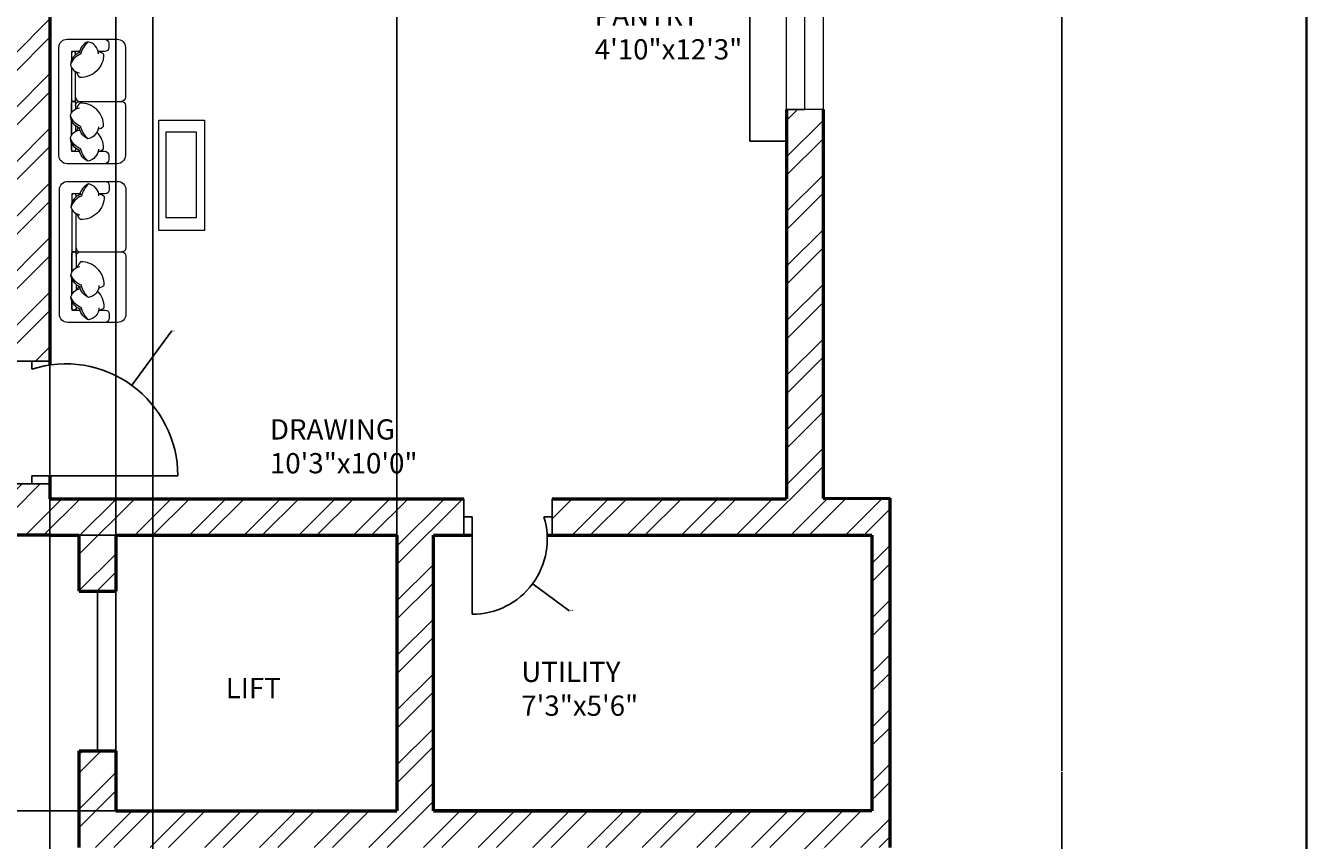
# Model space of a CAD drawing. Units: inches. Extents: x 1896 to 2572, y 1528 to 2474.
# Tile 9 of 10: x 2256 to 2572, y 2033 to 2234. Entities that reach past the tile are written whole.
import ezdxf

# ---------------------------------------------------------------- set-up
doc = ezdxf.new("R2010")
doc.units = ezdxf.units.IN
for name, color, linetype, lineweight in [('A-ANNO-DIMS', 2, 'Continuous', 18), ('A-ANNO-TTLB', 7, 'Continuous', 35), ('A-AREA-IDEN', 7, 'Continuous', 18), ('A-DOOR', 11, 'Continuous', 25), ('A-FLOR-CASE', 7, 'Continuous', 25), ('A-FURN', 8, 'Continuous', 18), ('A-GLAZ', 131, 'Continuous', 20), ('A-WALL', 7, 'Continuous', 50)]:
    doc.layers.add(name, color=color, linetype=linetype, lineweight=lineweight)
doc.layers.add('A-WALL-PATT', color=215, linetype='Continuous', lineweight=13, true_color=0xa953a0)
doc.styles.get("Standard").update_dxf_attribs({"font": 'arial.ttf'})
doc.dimstyles.get("Standard").update_dxf_attribs({"dimtxt": 0.18, "dimasz": 0.18, "dimexe": 0.18, "dimexo": 0.0625, "dimgap": 0.09, "dimtad": 0, "dimtih": 1, "dimtoh": 1, "dimdec": 4, "dimzin": 0, "dimdsep": 46, "dimtxsty": 'Standard', "dimcen": 0.09, "dimadec": 0, "dimazin": 0, "dimtfac": 1, "dimtdec": 4, "dimtofl": 0, "dimtmove": 0, "dimatfit": 3, "dimfxl": 1, "dimtolj": 1, "dimtzin": 0, "dimarcsym": 0})

# ---------------------------------------------------------------- blocks, each defined once
blk = doc.blocks.new('TABLE-COFFEE')
for points in [[(11.21, 0), (0, 0), (0, 27.27), (11.21, 27.27)], [(9.42, 2.87), (2.04, 2.87), (2.04, 24.13), (9.42, 24.13)]]:
    blk.add_lwpolyline(points, close=True)
blk = doc.blocks.new('WIN-36IN')
for p, q in [((0, 36), (9, 36)), ((0, 0), (0, 36)), ((9, 36), (4.5, 36)), ((4.5, 36), (4.5, 0)), ((9, 36), (9, 0)), ((4.5, 0), (0, 0)), ((0, 0), (9, 0))]:
    blk.add_line(p, q)
blk = doc.blocks.new('*D20')
at = {"layer": 'A-ANNO-DIMS', "color": 0, "lineweight": -2, "transparency": 16777216}
for p, q in [((2180.68, 2431.4), (2511.65, 2431.4)), ((2511.47, 2431.22), (2511.47, 2049.83)), ((2511.47, 1668.08), (2511.47, 2049.47)), ((2452.68, 1667.9), (2511.65, 1667.9))]:
    blk.add_line(p, q, dxfattribs=at)
at = {"layer": 'A-ANNO-DIMS', "color": 0, "transparency": 16777216}
for points in [[(2511.44, 2431.22), (2511.5, 2431.22), (2511.47, 2431.4)], [(2511.44, 1668.08), (2511.5, 1668.08), (2511.47, 1667.9)]]:
    blk.add_solid(points, dxfattribs=at)
at = {"layer": 'Defpoints', "color": 0, "transparency": 16777216}
for p in [(2180.62, 2431.4), (2511.47, 2431.4), (2452.62, 1667.9)]:
    blk.add_point(p, dxfattribs=at)
at = {"layer": 'A-ANNO-DIMS', "color": 0, "transparency": 16777216, "insert": (2511.47, 2049.65), "char_height": 0.18, "attachment_point": 5}
blk.add_mtext('\\A1;763.5', dxfattribs=at)
blk = doc.blocks.new('*D29')
at = {"layer": 'A-ANNO-DIMS', "color": 0, "lineweight": -2, "transparency": 16777216}
for p, q in [((2278.35, 2039.96), (2278.35, 2473.93)), ((2278.53, 2473.75), (2312.59, 2473.75)), ((2347.44, 2473.75), (2313.38, 2473.75)), ((2347.62, 2039.96), (2347.62, 2473.93))]:
    blk.add_line(p, q, dxfattribs=at)
at = {"layer": 'A-ANNO-DIMS', "color": 0, "transparency": 16777216}
for points in [[(2278.53, 2473.78), (2278.53, 2473.72), (2278.35, 2473.75)], [(2347.44, 2473.78), (2347.44, 2473.72), (2347.62, 2473.75)]]:
    blk.add_solid(points, dxfattribs=at)
at = {"layer": 'Defpoints', "color": 0, "transparency": 16777216}
for p in [(2347.62, 2473.75), (2278.35, 2039.9), (2347.62, 2039.9)]:
    blk.add_point(p, dxfattribs=at)
at = {"layer": 'A-ANNO-DIMS', "color": 0, "transparency": 16777216, "insert": (2312.99, 2473.75), "char_height": 0.18, "attachment_point": 5}
blk.add_mtext('\\A1;69.27', dxfattribs=at)
blk = doc.blocks.new('*D30')
at = {"layer": 'A-ANNO-DIMS', "color": 0, "lineweight": -2, "transparency": 16777216}
for p, q in [((2347.56, 2107.9), (1919.59, 2107.9)), ((1919.77, 2107.72), (1919.77, 2074.08)), ((1919.77, 2040.08), (1919.77, 2073.72)), ((2347.56, 2039.9), (1919.59, 2039.9))]:
    blk.add_line(p, q, dxfattribs=at)
at = {"layer": 'A-ANNO-DIMS', "color": 0, "transparency": 16777216}
for points in [[(1919.74, 2107.72), (1919.8, 2107.72), (1919.77, 2107.9)], [(1919.74, 2040.08), (1919.8, 2040.08), (1919.77, 2039.9)]]:
    blk.add_solid(points, dxfattribs=at)
at = {"layer": 'Defpoints', "color": 0, "transparency": 16777216}
for p in [(1919.77, 2107.9), (2347.62, 2107.9), (2347.62, 2039.9)]:
    blk.add_point(p, dxfattribs=at)
at = {"layer": 'A-ANNO-DIMS', "color": 0, "transparency": 16777216, "insert": (1919.77, 2073.9), "char_height": 0.18, "attachment_point": 5}
blk.add_mtext('\\A1;68', dxfattribs=at)
blk = doc.blocks.new('*D35')
at = {"layer": 'A-ANNO-DIMS', "color": 0, "lineweight": -2, "transparency": 16777216}
for p, q in [((2262.12, 2373.34), (2262.12, 1549.1)), ((2287.46, 2373.34), (2287.46, 1549.1)), ((2262.3, 1549.28), (2274.4, 1549.28)), ((2287.28, 1549.28), (2275.19, 1549.28))]:
    blk.add_line(p, q, dxfattribs=at)
at = {"layer": 'A-ANNO-DIMS', "color": 0, "transparency": 16777216}
for points in [[(2262.3, 1549.31), (2262.3, 1549.25), (2262.12, 1549.28)], [(2287.28, 1549.31), (2287.28, 1549.25), (2287.46, 1549.28)]]:
    blk.add_solid(points, dxfattribs=at)
at = {"layer": 'Defpoints', "color": 0, "transparency": 16777216}
for p in [(2262.12, 2373.4), (2287.46, 2373.4), (2287.46, 1549.28)]:
    blk.add_point(p, dxfattribs=at)
at = {"layer": 'A-ANNO-DIMS', "color": 0, "transparency": 16777216, "insert": (2274.79, 1549.28), "char_height": 0.18, "attachment_point": 5}
blk.add_mtext('\\A1;25.34', dxfattribs=at)
blk = doc.blocks.new('*D41')
at = {"layer": 'A-ANNO-DIMS', "color": 0, "lineweight": -2, "transparency": 16777216}
for p, q in [((2292.07, 2158.2), (2282.41, 2144.97)), ((2292.25, 2158.2), (2292.07, 2158.2)), ((2265.93, 2122.54), (2266.11, 2122.54)), ((2266.02, 2122.45), (2266.02, 2122.63))]:
    blk.add_line(p, q, dxfattribs=at)
at = {"layer": 'A-ANNO-DIMS', "color": 0, "transparency": 16777216}
blk.add_solid([(2282.38, 2144.99), (2282.43, 2144.96), (2282.3, 2144.83)], dxfattribs=at)
at = {"layer": 'Defpoints', "color": 0, "transparency": 16777216}
for p in [(2282.3, 2144.83), (2266.02, 2122.54)]:
    blk.add_point(p, dxfattribs=at)
at = {"layer": 'A-ANNO-DIMS', "color": 0, "transparency": 16777216, "insert": (2292.66, 2158.2), "char_height": 0.18, "attachment_point": 5}
blk.add_mtext('\\A1;R27.6', dxfattribs=at)
blk = doc.blocks.new('*D49')
at = {"layer": 'A-ANNO-DIMS', "color": 0, "lineweight": -2, "transparency": 16777216}
for p, q in [((2366.04, 2106.93), (2366.22, 2106.93)), ((2366.13, 2106.84), (2366.13, 2107.02)), ((2389.99, 2089.33), (2381.18, 2095.82)), ((2390.17, 2089.33), (2389.99, 2089.33))]:
    blk.add_line(p, q, dxfattribs=at)
at = {"layer": 'A-ANNO-DIMS', "color": 0, "transparency": 16777216}
blk.add_solid([(2381.2, 2095.85), (2381.17, 2095.8), (2381.04, 2095.93)], dxfattribs=at)
at = {"layer": 'Defpoints', "color": 0, "transparency": 16777216}
for p in [(2366.13, 2106.93), (2381.04, 2095.93)]:
    blk.add_point(p, dxfattribs=at)
at = {"layer": 'A-ANNO-DIMS', "color": 0, "transparency": 16777216, "insert": (2390.65, 2089.33), "char_height": 0.18, "attachment_point": 5}
blk.add_mtext('\\A1;R18.53', dxfattribs=at)

msp = doc.modelspace()

# ---------------------------------------------------------------- hatches: boundary and pattern name
at = {"layer": 'A-WALL-PATT'}
h = msp.add_hatch(dxfattribs=at)
h.set_pattern_fill('ANSI32', color=256)
h.paths.add_polyline_path([(2071.6224, 2382.3979), (2071.6224, 2422.3979), (2110.6224, 2422.3979), (2110.6224, 2382.3979), (2110.6224, 2357.5961), (2119.6224, 2357.5961), (2119.6224, 2422.3979), (2171.6224, 2422.3979), (2171.6224, 2373.3979), (2193.5093, 2373.3979), (2193.5093, 2377.8979), (2193.5093, 2382.3979), (2180.6224, 2382.3979), (2180.6224, 2431.3979), (2171.6224, 2431.3979), (2119.6224, 2431.3979), (2110.6224, 2431.3979), (2062.6224, 2431.3979), (2062.6224, 2422.3979), (2062.6224, 2382.3979), (1978.6224, 2382.3979), (1978.6224, 2313.0337), (1987.6224, 2313.0337), (1987.6224, 2373.3979), (2062.6224, 2373.3979), (2067.1224, 2373.3979), (2067.1224, 2353.7982), (2071.6224, 2353.8883)])
h.paths.add_polyline_path([(2287.4624, 2382.3979), (2229.5093, 2382.3979), (2229.5093, 2373.3979), (2253.1224, 2373.3979), (2253.1224, 2175.8979), (2247.1039, 2175.8979), (2247.1039, 2166.8979), (2253.1224, 2166.8979), (2253.1224, 2150.8283), (2262.1224, 2150.8283), (2262.1224, 2166.8979), (2262.1224, 2236.8979), (2349.0731, 2236.8979), (2349.0731, 2239.1479), (2349.0731, 2241.3979), (2262.1224, 2241.3979), (2262.1224, 2373.3979), (2287.4624, 2373.3979)])
h.paths.add_polyline_path([(2452.6224, 2382.3979), (2347.4624, 2382.3979), (2347.4624, 2373.3979), (2382.1224, 2373.3979), (2382.1224, 2334.0335), (2386.6224, 2334.0335), (2386.6224, 2373.3979), (2443.6224, 2373.3979), (2443.6224, 2316.2056), (2452.6224, 2316.2056)])
h.paths.add_polyline_path([(2452.6224, 2292.2056), (2448.1224, 2292.2056), (2443.6224, 2292.2056), (2443.6224, 2292.0047), (2443.6224, 2280.9372), (2443.6224, 2268.3979), (2386.6224, 2268.3979), (2386.6224, 2312.4044), (2384.3724, 2312.4044), (2382.1224, 2312.4044), (2382.1224, 2241.3979), (2379.1336, 2241.3979), (2379.1336, 2236.8979), (2386.6224, 2236.8979), (2386.6224, 2263.8979), (2443.6224, 2263.8979), (2443.6224, 2248.8449), (2452.6224, 2248.8449)])
h.paths.add_polyline_path([(2364.1285, 2116.8979), (2262.1224, 2116.8979), (2262.1224, 2120.5401), (2257.6224, 2120.5401), (2253.1224, 2120.5401), (2253.1224, 2107.8979), (2262.1224, 2107.8979), (2269.354, 2107.8979), (2269.354, 2094.0702), (2278.354, 2094.0702), (2278.354, 2107.8979), (2347.6224, 2107.8979), (2347.6224, 2039.8979), (2278.354, 2039.8979), (2278.354, 2054.7605), (2269.354, 2054.7605), (2269.354, 2030.8979), (2278.354, 2030.8979), (2443.6224, 2030.8979), (2443.6224, 2015.198), (2452.6224, 2015.198), (2452.6224, 2030.8979), (2464.6224, 2030.8979), (2469.1224, 2030.8979), (2469.1224, 2117.0352), (2452.6767, 2116.9466), (2452.6285, 2125.8979), (2452.6224, 2125.8979), (2452.6224, 2212.8449), (2443.6224, 2212.8449), (2443.6224, 2116.8979), (2385.832, 2116.8979), (2385.832, 2112.3979), (2385.832, 2107.8979), (2464.6224, 2107.8979), (2464.6224, 2039.8979), (2443.6224, 2039.8979), (2356.6224, 2039.8979), (2356.6224, 2107.8979), (2364.1285, 2107.8979)])
h.paths.add_polyline_path([(2452.6224, 1967.198), (2443.6224, 1967.198), (2443.6224, 1955.8979), (2259.1224, 1955.8979), (2254.6224, 1955.8979), (2254.6224, 1941.6358), (2263.6224, 1941.6358), (2263.6224, 1946.8979), (2379.1224, 1946.8979), (2379.1224, 1913.0204), (2383.6224, 1913.0204), (2383.6224, 1946.8979), (2443.6224, 1946.8979), (2443.6224, 1930.729), (2452.6224, 1930.729)])
h.paths.add_polyline_path([(2469.1224, 1871.8979), (2464.6224, 1871.8979), (2452.6224, 1871.8979), (2452.6224, 1894.729), (2443.6224, 1894.729), (2443.6224, 1871.8979), (2388.1304, 1871.8979), (2388.1304, 1867.3979), (2443.6224, 1867.3979), (2464.6224, 1867.3979), (2464.6224, 1817.8979), (2443.6224, 1817.8979), (2388.1304, 1817.8979), (2388.1304, 1815.6479), (2388.1304, 1813.3979), (2391.1224, 1813.3979), (2391.1224, 1747.8899), (2395.6224, 1747.8899), (2395.6224, 1813.3979), (2443.6224, 1813.3979), (2443.6224, 1781.4434), (2452.6224, 1781.4434), (2452.6224, 1813.3979), (2464.6224, 1813.3979), (2469.1224, 1813.3979)])
h.paths.add_polyline_path([(2263.6224, 1910.9737), (2259.1224, 1910.9737), (2254.6224, 1910.9737), (2254.6224, 1889.8979), (2251.2778, 1889.8979), (2251.2778, 1880.8979), (2254.6224, 1880.8979), (2254.6224, 1817.8979), (2254.6224, 1754.8979), (2254.6224, 1693.3979), (2254.6224, 1684.3979), (2254.6224, 1672.3979), (2200.6224, 1672.3979), (2200.6224, 1684.3979), (2200.6224, 1693.3979), (2200.6224, 1754.8979), (2196.1224, 1754.8979), (2196.1224, 1693.3979), (2150.0488, 1693.3979), (2150.0488, 1684.3979), (2196.1224, 1684.3979), (2196.1224, 1672.3979), (2196.1224, 1667.8979), (2254.6224, 1667.8979), (2259.1224, 1667.8979), (2259.1224, 1693.3979), (2259.1224, 1813.3979), (2353.6224, 1813.3979), (2353.6224, 1815.6479), (2353.6224, 1817.8979), (2263.6224, 1817.8979)])
h.paths.add_polyline_path([(2391.1224, 1693.3979), (2345.6981, 1693.3979), (2345.6981, 1684.3979), (2391.1224, 1684.3979)])
h.paths.add_polyline_path([(2285.6981, 1693.3979), (2259.1224, 1693.3979), (2259.1224, 1684.3979), (2285.6981, 1684.3979), (2285.6981, 1688.8979)], flags=17)
h.paths.add_polyline_path([(2452.6224, 1757.4434), (2448.1224, 1757.4434), (2443.6224, 1757.4434), (2443.6224, 1726.3979), (2395.6224, 1726.3979), (2395.6224, 1728.6572), (2393.3724, 1728.6572), (2391.1224, 1728.6572), (2391.1224, 1717.6723), (2395.6224, 1717.6723), (2395.6224, 1721.8979), (2443.6224, 1721.8979), (2443.6224, 1714.8), (2452.6224, 1714.8)])
h.paths.add_polyline_path([(2452.6224, 1684.3979), (2452.6224, 1690.8), (2443.6224, 1690.8), (2443.6224, 1679.8979), (2443.6224, 1672.3979), (2395.6224, 1672.3979), (2395.6224, 1695.6708), (2391.1224, 1695.5986), (2391.1224, 1672.3979), (2391.1224, 1667.8979), (2452.6224, 1667.8979)])
h.paths.add_polyline_path([(1987.6224, 1880.8979), (2068.6224, 1880.8979), (2125.6224, 1880.8979), (2125.6224, 1788.8466), (2130.1224, 1788.8466), (2130.1224, 1880.8979), (2216.1958, 1880.8979), (2216.1958, 1885.3979), (2216.1958, 1889.8979), (2208.1224, 1889.8979), (2208.1224, 1996.3717), (2203.6224, 1996.3717), (2199.1224, 1996.3717), (2199.1224, 1889.8979), (2073.1224, 1889.8979), (2073.1224, 1917.1874), (2068.6224, 1917.1874), (2068.6224, 1889.8979), (1987.6224, 1889.8979), (1987.6224, 1912.4976), (1978.6224, 1912.4976), (1978.6224, 1805.5193), (1987.6224, 1805.5193)])
h.paths.add_polyline_path([(2019.9303, 1754.8979), (1987.6224, 1754.8979), (1966.6224, 1754.8979), (1966.6224, 1801.0193), (1987.6224, 1801.0193), (1987.6224, 1805.5193), (1962.1224, 1805.5193), (1962.1224, 1750.3979), (1966.6224, 1750.3979), (1978.6224, 1750.3979), (1987.6224, 1750.3979), (2019.9303, 1750.3979)])
h.paths.add_polyline_path([(2135.5566, 1754.8979), (2130.1224, 1754.8979), (2130.1224, 1758.052), (2127.8724, 1758.052), (2125.6224, 1758.052), (2125.6224, 1754.8979), (2068.6224, 1754.8979), (2043.2292, 1754.8979), (2043.2292, 1750.3979), (2068.6224, 1750.3979), (2098.6224, 1750.3979), (2098.6224, 1693.3979), (2068.6224, 1693.3979), (1987.6224, 1693.3979), (1987.6224, 1707.3003), (1983.1224, 1707.3003), (1978.6224, 1707.3003), (1978.6224, 1684.3979), (2068.6224, 1684.3979), (2126.0488, 1684.3979), (2126.0488, 1688.8979), (2126.0488, 1693.3979), (2103.1224, 1693.3979), (2103.1224, 1750.3979), (2130.1224, 1750.3979), (2135.5566, 1750.3979)])
h.paths.add_polyline_path([(1987.6224, 1750.3979), (1978.6224, 1750.3979), (1978.6224, 1731.3003), (1987.6224, 1731.3003)], flags=0)
h.paths.add_polyline_path([(1987.6224, 1973.8979), (2068.6224, 1973.8979), (2073.1224, 1973.8979), (2073.1224, 1978.3979), (1971.1224, 1978.3979), (1971.1224, 2030.3979), (1978.6224, 2030.3979), (1987.6224, 2030.3979), (2104.9199, 2030.3979), (2104.9199, 2032.6479), (2104.9199, 2034.8979), (1987.6224, 2034.8979), (1971.1224, 2034.8979), (1971.1224, 2085.8979), (2003.6464, 2085.8979), (2003.6464, 2090.3979), (1987.6224, 2090.3979), (1987.6224, 2166.8979), (2115.1224, 2166.8979), (2137.6224, 2166.8979), (2137.6224, 2114.4229), (2142.1224, 2114.4229), (2142.1224, 2124.8979), (2153.5306, 2124.8979), (2153.5306, 2127.1479), (2153.5306, 2129.3979), (2142.1224, 2129.3979), (2142.1224, 2166.8979), (2199.1224, 2166.8979), (2199.1224, 2129.3979), (2177.5306, 2129.3979), (2177.5306, 2124.8979), (2199.1224, 2124.8979), (2199.1224, 2034.8979), (2142.1224, 2034.8979), (2142.1224, 2091.6671), (2139.8724, 2091.6671), (2137.6224, 2091.6671), (2137.6224, 2034.8979), (2133.8326, 2034.8979), (2133.8326, 2030.3979), (2137.6224, 2030.3979), (2142.1224, 2030.3979), (2199.1224, 2030.3979), (2199.1224, 2024.2654), (2208.1224, 2024.2654), (2208.1224, 2030.3979), (2208.1224, 2166.8979), (2214.5775, 2166.8979), (2214.5775, 2171.3979), (2214.5775, 2175.8979), (2115.1224, 2175.8979), (2115.1224, 2329.9154), (2112.4137, 2329.9154), (2110.6224, 2329.9154), (2110.6224, 2175.8979), (2082.1224, 2175.8979), (2082.1224, 2202.6443), (2079.8724, 2202.6443), (2077.6224, 2202.6443), (2077.6224, 2175.8979), (1987.6224, 2175.8979), (1987.6224, 2191.3531), (1983.1224, 2191.3531), (1978.6224, 2191.3531), (1978.6224, 2090.3979), (1966.6224, 2090.3979), (1966.6224, 2085.8979), (1966.6224, 2030.3979), (1966.6224, 1973.8979), (1978.6224, 1973.8979), (1978.6224, 1948.4976), (1983.1224, 1948.4976), (1987.6224, 1948.4976)])
h.paths.add_polyline_path([(1987.6224, 2253.0337), (1983.1224, 2253.0337), (1978.6224, 2253.0337), (1978.6224, 2215.3531), (1987.6224, 2215.3531), (1987.6224, 2224.8979), (2077.6224, 2224.8979), (2077.6224, 2221.9854), (2082.1224, 2221.9854), (2082.1224, 2229.3979), (1987.6224, 2229.3979)], flags=17)
h.paths.add_polyline_path([(2220.5047, 1978.7278), (2253.7278, 1978.7278), (2253.7278, 1997.3851), (2220.5047, 1997.3851)], flags=9)
h.paths.add_polyline_path([(2303.6746, 2064.9806), (2320.5334, 2064.9806), (2320.5334, 2075.2842), (2303.6746, 2075.2842)], flags=25)

# ---------------------------------------------------------------- linework, layer by layer
at = {"layer": 'A-ANNO-TTLB'}
msp.add_lwpolyline([(1895.84, 2455.9668), (2571.702, 2455.9668), (2571.702, 1527.8833), (1895.84, 1527.8833)], close=True, dxfattribs=at)
at = {"layer": 'A-DOOR'}
for p, q in [((2253.1224, 2150.8283), (2262.1224, 2150.8283)), ((2262.1224, 2150.8283), (2257.6224, 2150.8283)), ((2257.6224, 2150.8283), (2257.6224, 2148.8283)), ((2257.6224, 2120.5401), (2257.6224, 2122.5401)), ((2257.6224, 2122.5401), (2293.6224, 2122.5401)), ((2253.1224, 2120.5401), (2262.1224, 2120.5401)), ((2262.1224, 2120.5401), (2257.6224, 2120.5401)), ((2364.1285, 2107.8979), (2364.1285, 2116.8979)), ((2364.1285, 2116.8979), (2364.1285, 2112.3979)), ((2385.832, 2107.8979), (2385.832, 2116.8979)), ((2385.832, 2116.8979), (2385.832, 2116.8979)), ((2385.832, 2116.8979), (2385.832, 2112.3979)), ((2364.1285, 2112.3979), (2366.1285, 2112.3979)), ((2366.1285, 2112.3979), (2366.1285, 2088.3979)), ((2385.832, 2112.3979), (2383.832, 2112.3979)), ((2273.854, 2094.0702), (2273.854, 2054.7605))]:
    msp.add_line(p, q, dxfattribs=at)
for centre, radius, start, end in [((2266.0243, 2122.5401), 27.5982, 0, 107.724107), ((2366.1285, 2106.9274), 18.5295, 270, 17.171415)]:
    msp.add_arc(centre, radius, start, end, dxfattribs=at)
at = {"layer": 'A-FLOR-CASE'}
for p, q in [((2434.5516, 2255.5451), (2434.5516, 2205.0449)), ((2434.5516, 2205.0449), (2443.6224, 2205.0449))]:
    msp.add_line(p, q, dxfattribs=at)
at = {"layer": 'A-FURN', "ltscale": 0.03}
for points in [[(2280.7017, 2215.8729, -0.41421356), (2279.6783, 2214.8495, -0.41421356), (2280.7017, 2213.8261), (2280.7017, 2201.5452, -0.41421356), (2278.6549, 2199.4984), (2266.374, 2199.4984, -0.41421356), (2264.3272, 2201.5452), (2264.3272, 2228.1538, -0.41421356), (2266.374, 2230.2006), (2278.6549, 2230.2006, -0.41421356), (2280.7017, 2228.1538), (2280.7017, 2215.8729, -0.41421356), (2279.6783, 2214.8495, -0.41421356), (2280.7017, 2213.8261)], [(2280.8392, 2178.7738, -0.41421356), (2279.8158, 2177.7504, -0.41421356), (2280.8392, 2176.727), (2280.8392, 2162.3993, -0.41421356), (2278.7924, 2160.3525), (2266.5115, 2160.3525, -0.41421356), (2264.4647, 2162.3993), (2264.4647, 2193.1016, -0.41421356), (2266.5115, 2195.1484), (2278.7924, 2195.1484, -0.41421356), (2280.8392, 2193.1016), (2280.8392, 2178.7738, -0.41421356), (2279.8158, 2177.7504, -0.41421356), (2280.8392, 2176.727)]]:
    msp.add_lwpolyline(points, format="xyb", dxfattribs=at)
at = {"layer": 'A-FURN'}
for points in [[(2271.4814, 2229.5493, 0.14772988), (2269.7225, 2226.5581, 0.21334276), (2267.1429, 2223.9189, 0.17866181)], [(2274.061, 2226.6168, 0.35677236), (2271.4814, 2229.5493, 0.24954205), (2269.3555, 2226.8922, -9.61688035)], [(2275.5847, 2230.2006, -0.41421356), (2276.6081, 2229.1772), (2276.6081, 2228.1538, -0.41421356), (2275.5847, 2227.1304), (2273.9991, 2227.1304)], [(2269.5824, 2226.9714, 0.30666349), (2267.1429, 2223.9189, 0.30632997), (2269.3708, 2221.9248, -0.87284716)], [(2268.4208, 2226.3494), (2268.4208, 2226.721, 0.41421356), (2268.0115, 2227.1304), (2267.8068, 2227.1304, 0.41421356), (2267.3974, 2226.721)], [(2267.3974, 2226.721), (2267.3974, 2224.9774, 0.41421356)], [(2273.9986, 2227.1326, -0.16554063), (2275.3508, 2226.4995, -0.42598917), (2269.488, 2220.7518, -0.12152332), (2268.68, 2222.1162, 7.11546429)], [(2267.3974, 2223.2748), (2267.3974, 2215.2589, 0.41421356), (2267.8068, 2214.8495), (2268.0115, 2214.8495, 0.41421356), (2268.4208, 2215.2589), (2268.4208, 2222.2443, 0.41421356)], [(2268.4208, 2215.8729, 0.41421356), (2269.4442, 2214.8495)], [(2268.4208, 2215.8729, 0.41421356), (2269.4442, 2214.8495), (2279.6783, 2214.8495, 0.41421356)], [(2269.5824, 2208.2407, -0.30666349), (2267.1429, 2211.2931, -0.30632997), (2269.3708, 2213.2872, 0.87284716)], [(2267.3974, 2211.9372), (2267.3974, 2214.4401, -0.41421356), (2267.8068, 2214.8495), (2268.0115, 2214.8495, -0.41421356), (2268.4208, 2214.4401), (2268.4208, 2212.9677, -0.41421356)], [(2268.4208, 2213.8261, -0.41421356), (2269.4442, 2214.8495)], [(2268.4208, 2213.8261, -0.41421356), (2269.4442, 2214.8495), (2279.6783, 2214.8495, -0.41421356)], [(2273.9986, 2208.0794, 0.16554063), (2275.3508, 2208.7125, 0.42598917), (2269.488, 2214.4602, 0.12152332), (2268.68, 2213.0958, -7.11546429)], [(2271.4814, 2205.6628, -0.14772988), (2269.7225, 2208.6539, -0.21334276), (2267.1429, 2211.2931, -0.17866181)], [(2267.3974, 2206.4241), (2267.3974, 2210.2346, -0.41421356)], [(2269.5824, 2202.7276, -0.30666349), (2267.1429, 2205.7801, -0.30632997), (2269.3708, 2207.7742, 0.87284716)], [(2268.4208, 2208.8626), (2268.4208, 2207.4547, -0.41421356)], [(2269.0801, 2208.4408, 0.07186538), (2268.68, 2207.5828, -7.11546429)], [(2274.061, 2208.5952, -0.35677236), (2271.4814, 2205.6628, -0.24954205), (2269.3555, 2208.3199, 9.61688035)], [(2273.9986, 2202.5664, 0.16554063), (2275.3508, 2203.1995, 0.20023115), (2273.7039, 2207.262, 0.12152332)], [(2271.4814, 2200.1497, -0.14772988), (2269.7225, 2203.1408, -0.21334276), (2267.1429, 2205.7801, -0.17866181)], [(2267.3974, 2202.978), (2267.3974, 2204.7216, -0.41421356)], [(2267.3974, 2204.7216), (2267.3974, 2202.5686), (2269.4087, 2202.5686, -0.41421356)], [(2268.4208, 2203.3496), (2268.4208, 2202.978, -0.41421356), (2268.0115, 2202.5686), (2267.8068, 2202.5686, -0.41421356), (2267.3974, 2202.978)], [(2274.061, 2203.0822, -0.35677236), (2271.4814, 2200.1497, -0.24954205), (2269.3555, 2202.8068, 9.61688035)], [(2273.9991, 2202.5686), (2275.5847, 2202.5686, -0.41421356), (2276.6081, 2201.5452), (2276.6081, 2200.5218, -0.41421356), (2275.5847, 2199.4984)], [(2271.6189, 2194.497, 0.14772988), (2269.86, 2191.5059, 0.21334276), (2267.2804, 2188.8667, 0.17866181)], [(2274.1985, 2191.5646, 0.35677236), (2271.6189, 2194.497, 0.24954205), (2269.493, 2191.8399, -9.61688035)], [(2275.7222, 2195.1484, -0.41421356), (2276.7456, 2194.125), (2276.7456, 2193.1016, -0.41421356), (2275.7222, 2192.0781), (2274.1365, 2192.0781)], [(2269.7199, 2191.9191, 0.30666349), (2267.2804, 2188.8667, 0.30632997), (2269.5083, 2186.8726, -0.87284716)], [(2268.5583, 2191.2972), (2268.5583, 2191.6688, 0.41421356), (2268.149, 2192.0781), (2267.9443, 2192.0781, 0.41421356), (2267.5349, 2191.6688)], [(2267.5349, 2191.6688), (2267.5349, 2189.9252, 0.41421356)], [(2274.1361, 2192.0804, -0.16554063), (2275.4883, 2191.4473, -0.42598917), (2269.6255, 2185.6996, -0.12152332), (2268.8174, 2187.064, 7.11546429)], [(2267.5349, 2188.2226), (2267.5349, 2178.1598, 0.41421356), (2267.9443, 2177.7504), (2268.149, 2177.7504, 0.41421356), (2268.5583, 2178.1598), (2268.5583, 2187.1921, 0.41421356)], [(2267.5349, 2172.7913), (2267.5349, 2177.3411, -0.41421356), (2267.9443, 2177.7504), (2268.149, 2177.7504, -0.41421356), (2268.5583, 2177.3411), (2268.5583, 2173.8218, -0.41421356)], [(2268.5583, 2178.7738, 0.41421356), (2269.5817, 2177.7504)], [(2268.5583, 2178.7738, 0.41421356), (2269.5817, 2177.7504), (2279.8158, 2177.7504, 0.41421356)], [(2268.5583, 2176.727, -0.41421356), (2269.5817, 2177.7504)], [(2268.5583, 2176.727, -0.41421356), (2269.5817, 2177.7504), (2279.8158, 2177.7504, -0.41421356)], [(2274.1361, 2168.9336, 0.16554063), (2275.4883, 2169.5667, 0.42598917), (2269.6255, 2175.3143, 0.12152332), (2268.8174, 2173.9499, -7.11546429)], [(2269.7199, 2169.0948, -0.30666349), (2267.2804, 2172.1473, -0.30632997), (2269.5083, 2174.1413, 0.87284716)], [(2271.6189, 2166.5169, -0.14772988), (2269.86, 2169.508, -0.21334276), (2267.2804, 2172.1473, -0.17866181)], [(2269.7199, 2163.5817, -0.30666349), (2267.2804, 2166.6342, -0.30632997), (2269.5083, 2168.6283, 0.87284716)], [(2267.5349, 2167.2783), (2267.5349, 2171.0888, -0.41421356)], [(2268.5583, 2169.7168), (2268.5583, 2168.3088, -0.41421356)], [(2269.2175, 2169.2949, 0.07186538), (2268.8174, 2168.4369, -7.11546429)], [(2274.1985, 2169.4494, -0.35677236), (2271.6189, 2166.5169, -0.24954205), (2269.493, 2169.174, 9.61688035)], [(2274.1361, 2163.4205, 0.16554063), (2275.4883, 2164.0536, 0.20023115), (2273.8414, 2168.1162, 0.12152332)], [(2271.6189, 2161.0038, -0.14772988), (2269.86, 2163.995, -0.21334276), (2267.2804, 2166.6342, -0.17866181)], [(2267.5349, 2165.5757), (2267.5349, 2163.4227), (2269.5462, 2163.4227, -0.41421356)], [(2267.5349, 2163.8321), (2267.5349, 2165.5757, -0.41421356)], [(2268.5583, 2164.2037), (2268.5583, 2163.8321, -0.41421356), (2268.149, 2163.4227), (2267.9443, 2163.4227, -0.41421356), (2267.5349, 2163.8321)], [(2274.1985, 2163.9363, -0.35677236), (2271.6189, 2161.0038, -0.24954205), (2269.493, 2163.6609, 9.61688035)], [(2274.1365, 2163.4227), (2275.7222, 2163.4227, -0.41421356), (2276.7456, 2162.3993), (2276.7456, 2161.3759, -0.41421356), (2275.7222, 2160.3525)]]:
    msp.add_lwpolyline(points, format="xyb", dxfattribs=at)
for points in [[(2269.4087, 2227.1304), (2267.3974, 2227.1304), (2267.3974, 2224.9774)], [(2267.3974, 2223.2748), (2267.3974, 2211.9372)], [(2267.3974, 2210.2346), (2267.3974, 2206.4241)], [(2269.5462, 2192.0781), (2267.5349, 2192.0781), (2267.5349, 2189.9252)], [(2267.5349, 2188.2226), (2267.5349, 2172.7913)], [(2267.5349, 2171.0888), (2267.5349, 2167.2783)]]:
    msp.add_lwpolyline(points, dxfattribs=at)
for points in [[(2267.3974, 2215.2589), (2267.3974, 2214.4401, -0.41421356), (2267.8068, 2214.8495), (2268.0115, 2214.8495, -0.41421356), (2268.4208, 2214.4401), (2268.4208, 2215.2589, -0.41421356), (2268.0115, 2214.8495), (2267.8068, 2214.8495, -0.41421356)], [(2267.5349, 2178.1598), (2267.5349, 2177.3411, -0.41421356), (2267.9443, 2177.7504), (2268.149, 2177.7504, -0.41421356), (2268.5583, 2177.3411), (2268.5583, 2178.1598, -0.41421356), (2268.149, 2177.7504), (2267.9443, 2177.7504, -0.41421356)]]:
    msp.add_lwpolyline(points, format="xyb", close=True, dxfattribs=at)
at = {"layer": 'A-WALL'}
for p, q in [((2262.1224, 2236.8979), (2262.1224, 2166.8979)), ((2443.6224, 2212.8449), (2443.6224, 2116.8979)), ((2452.6224, 2212.8449), (2452.6224, 2125.8979)), ((2262.1224, 2166.8979), (2262.1224, 2149.861)), ((2452.6224, 2127.0186), (2452.6767, 2116.9466)), ((2452.6285, 2125.8979), (2452.6224, 2125.8979)), ((2262.1224, 2122.5401), (2262.1224, 2116.8979)), ((2262.1224, 2116.8979), (2364.1285, 2116.8979)), ((2385.832, 2116.8979), (2443.6224, 2116.8979)), ((2452.6767, 2116.9466), (2469.1224, 2117.0352)), ((2469.1224, 2116.8979), (2469.1224, 2117.0352)), ((2469.1224, 2030.8979), (2469.1224, 2116.8979)), ((2262.1224, 2107.8979), (2253.1224, 2107.8979)), ((2262.1224, 2107.8979), (2269.354, 2107.8979)), ((2269.354, 2094.0702), (2269.354, 2107.8979)), ((2278.354, 2107.8979), (2278.354, 2094.0702)), ((2278.354, 2107.8979), (2347.6224, 2107.8979)), ((2347.6224, 2107.8979), (2347.6224, 2039.8979)), ((2356.6224, 2039.8979), (2356.6224, 2107.8979)), ((2356.6224, 2107.8979), (2366.1285, 2107.8979)), ((2384.6325, 2107.8979), (2464.6224, 2107.8979)), ((2464.6224, 2107.8979), (2464.6224, 2039.8979)), ((2269.354, 2094.0702), (2278.354, 2094.0702)), ((2269.354, 2030.8979), (2269.354, 2054.7605)), ((2269.354, 2054.7605), (2278.354, 2054.7605)), ((2278.354, 2054.7605), (2278.354, 2039.8979)), ((2278.354, 2039.8979), (2347.6224, 2039.8979)), ((2443.6224, 2039.8979), (2356.6224, 2039.8979)), ((2356.6224, 2039.8979), (2443.6224, 2039.8979)), ((2464.6224, 2039.8979), (2443.6224, 2039.8979))]:
    msp.add_line(p, q, dxfattribs=at)

# ---------------------------------------------------------------- block references
at = {"layer": 'A-FURN', "rotation": 180}
msp.add_blockref('TABLE-COFFEE', (2300.1934, 2210.2606), dxfattribs=at)
at = {"layer": 'A-GLAZ', "rotation": 180}
msp.add_blockref('WIN-36IN', (2452.6229, 2248.8449), dxfattribs=at)

# ---------------------------------------------------------------- texts
at = {"layer": 'A-AREA-IDEN', "char_height": 5, "attachment_point": 1}
for s, width, insert in [('PANTRY\\P4\'10"x12\'3"', 78.851393, (2396.3448, 2238.53)), ('DRAWING\\P10\'3"x10\'0"', 206.306014, (2316.3204, 2136.4849)), ('UTILITY\\P7\'3"x5\'6"', 155.37841, (2378.2574, 2076.7056)), ('LIFT', 94.957629, (2305.4362, 2072.7108))]:
    msp.add_mtext_dynamic_manual_height_columns(s, width=width, gutter_width=12.5, heights=[0], dxfattribs=dict(at, insert=insert))

# ---------------------------------------------------------------- dimensions: what is measured, and where the dimension line sits
at = {"layer": 'A-ANNO-DIMS'}
for base, p1, p2, picture, middle in [((2347.6224, 2473.7479), (2278.354, 2039.8979), (2347.6224, 2039.8979), '*D29', (2312.9882, 2473.7479)), ((2287.4624, 1549.2803), (2262.1224, 2373.3979), (2287.4624, 2373.3979), '*D35', (2274.7924, 1549.2803))]:
    dim = msp.add_linear_dim(base=base, p1=p1, p2=p2, dimstyle='Standard', override={"dimdec": 2, "dimlfac": 1, "dimrnd": 0, "dimzin": 0, "dimdsep": 46, "dimlunit": 2}, dxfattribs=at)
    dim.commit()
    dim.dimension.update_dxf_attribs({"geometry": picture, "text_midpoint": middle})
for base, p1, p2, override, picture, middle in [((2511.4724, 2431.3979), (2452.6224, 1667.8979), (2180.6224, 2431.3979), {"dimdec": 1, "dimlfac": 1, "dimrnd": 0, "dimzin": 0, "dimdsep": 46, "dimlunit": 2}, '*D20', (2511.4724, 2049.6479)), ((1919.7724, 2107.8979), (2347.6224, 2039.8979), (2347.6224, 2107.8979), {"dimdec": 0, "dimlfac": 1, "dimrnd": 0, "dimzin": 0, "dimdsep": 46, "dimlunit": 2}, '*D30', (1919.7724, 2073.8979))]:
    dim = msp.add_linear_dim(base=base, p1=p1, p2=p2, angle=90, dimstyle='Standard', override=override, dxfattribs=at)
    dim.commit()
    dim.dimension.update_dxf_attribs({"geometry": picture, "text_midpoint": middle})
for center, mpoint, override, picture, middle in [((2266.0243, 2122.5401), (2282.3001, 2144.8281), {"dimdec": 1, "dimlfac": 1, "dimrnd": 0, "dimzin": 0, "dimdsep": 46, "dimlunit": 2}, '*D41', (2292.6554, 2158.2009)), ((2366.1285, 2106.9274), (2381.0401, 2095.928), {"dimdec": 2, "dimlfac": 1, "dimrnd": 0, "dimzin": 0, "dimdsep": 46, "dimlunit": 2}, '*D49', (2390.6468, 2089.3283))]:
    dim = msp.add_radius_dim(center=center, mpoint=mpoint, dimstyle='Standard', override=override, dxfattribs=at)
    dim.commit()
    dim.dimension.update_dxf_attribs({"geometry": picture, "text_midpoint": middle, "dimtype": 164})

doc.saveas('drawing.dxf')
